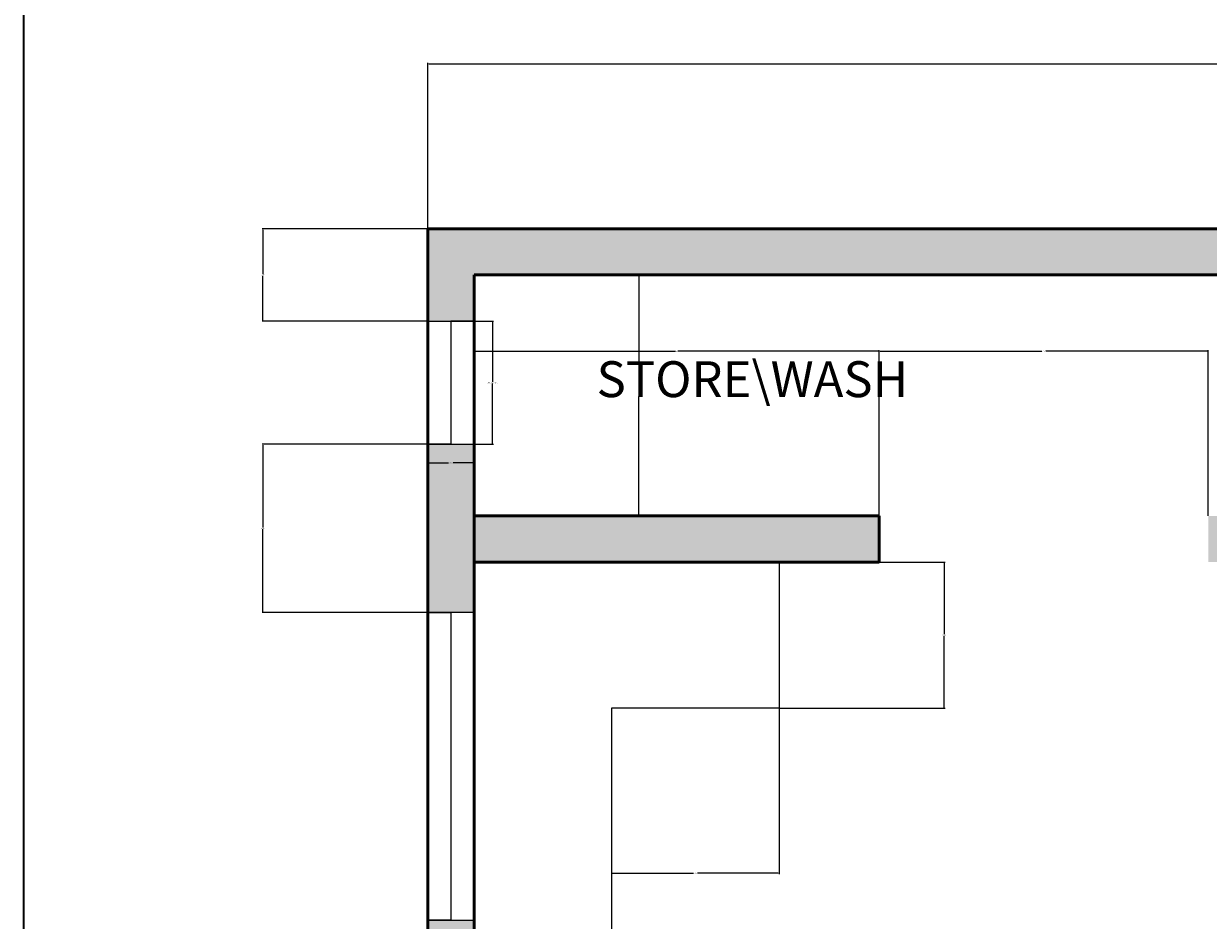
# Model space of a CAD drawing. Units: inches. Extents: x 1676 to 2199, y 1657 to 2783.
# Tile 6 of 10: x 1676 to 1907, y 2206 to 2381. Entities that reach past the tile are written whole.
import ezdxf

# ---------------------------------------------------------------- set-up
doc = ezdxf.new("R2010")
doc.units = ezdxf.units.IN
for name, color, linetype, lineweight in [('A-ANNO-DIMS', 2, 'Continuous', 18), ('A-ANNO-TTLB', 7, 'Continuous', 35), ('A-AREA-IDEN', 7, 'Continuous', 18), ('A-FLOR-CASE', 7, 'Continuous', 25), ('A-GLAZ', 4, 'Continuous', 18), ('A-WALL', 7, 'Continuous', 50)]:
    doc.layers.add(name, color=color, linetype=linetype, lineweight=lineweight)
doc.layers.add('A-WALL-PATT', color=251, linetype='Continuous', lineweight=13, true_color=0x636466)
doc.styles.get("Standard").update_dxf_attribs({"font": 'arial.ttf'})
doc.dimstyles.get("Standard").update_dxf_attribs({"dimtxt": 0.18, "dimasz": 0.18, "dimexe": 0.18, "dimexo": 0.0625, "dimgap": 0.09, "dimtad": 0, "dimtih": 1, "dimtoh": 1, "dimdec": 4, "dimzin": 0, "dimdsep": 46, "dimtxsty": 'Standard', "dimcen": 0.09, "dimadec": 0, "dimazin": 0, "dimtfac": 1, "dimtdec": 4, "dimtofl": 0, "dimtmove": 0, "dimatfit": 3, "dimfxl": 1, "dimtolj": 1, "dimtzin": 0, "dimarcsym": 0})

# ---------------------------------------------------------------- blocks, each defined once
blk = doc.blocks.new('WIN-24')
for p, q in [((0, 0), (9, 0)), ((9, 0), (4.5, 0)), ((4.5, 0), (4.5, -24)), ((4.5, -24), (0, -24)), ((0, -24), (9, -24))]:
    blk.add_line(p, q)
blk = doc.blocks.new('*D9')
at = {"layer": 'A-ANNO-DIMS', "color": 0, "lineweight": -2, "transparency": 16777216}
for p, q in [((1764.14, 2323.07), (1767.85, 2323.07)), ((1767.67, 2322.89), (1767.67, 2311.26)), ((1767.67, 2299.25), (1767.67, 2310.89)), ((1764.14, 2299.07), (1767.85, 2299.07))]:
    blk.add_line(p, q, dxfattribs=at)
at = {"layer": 'A-ANNO-DIMS', "color": 0, "transparency": 16777216}
for points in [[(1767.64, 2322.89), (1767.7, 2322.89), (1767.67, 2323.07)], [(1767.64, 2299.25), (1767.7, 2299.25), (1767.67, 2299.07)]]:
    blk.add_solid(points, dxfattribs=at)
at = {"layer": 'Defpoints', "color": 0, "transparency": 16777216}
for p in [(1764.07, 2323.07), (1767.67, 2323.07), (1764.07, 2299.07)]:
    blk.add_point(p, dxfattribs=at)
at = {"layer": 'A-ANNO-DIMS', "color": 0, "transparency": 16777216, "insert": (1767.67, 2311.07), "char_height": 0.18, "attachment_point": 5}
blk.add_mtext('\\A1;WINDOW 24 TYP.', dxfattribs=at)
blk = doc.blocks.new('*D10')
at = {"layer": 'A-ANNO-DIMS', "color": 0, "lineweight": -2, "transparency": 16777216}
for p, q in [((1755.07, 2299.01), (1755.07, 2295.29)), ((1764.07, 2299.01), (1764.07, 2295.29)), ((1755.25, 2295.47), (1759.12, 2295.47)), ((1763.89, 2295.47), (1760.03, 2295.47))]:
    blk.add_line(p, q, dxfattribs=at)
at = {"layer": 'A-ANNO-DIMS', "color": 0, "transparency": 16777216}
for points in [[(1755.25, 2295.5), (1755.25, 2295.44), (1755.07, 2295.47)], [(1763.89, 2295.5), (1763.89, 2295.44), (1764.07, 2295.47)]]:
    blk.add_solid(points, dxfattribs=at)
at = {"layer": 'Defpoints', "color": 0, "transparency": 16777216}
for p in [(1755.07, 2299.07), (1764.07, 2299.07), (1764.07, 2295.47)]:
    blk.add_point(p, dxfattribs=at)
at = {"layer": 'A-ANNO-DIMS', "color": 0, "transparency": 16777216, "insert": (1759.57, 2295.47), "char_height": 0.18, "attachment_point": 5}
blk.add_mtext('\\A1;9 TYP.', dxfattribs=at)
blk = doc.blocks.new('*D19')
at = {"layer": 'A-ANNO-DIMS', "color": 0, "lineweight": -2, "transparency": 16777216}
for p, q in [((1755.07, 2341.15), (1755.07, 2373.42)), ((1755.25, 2373.24), (1948.29, 2373.24)), ((2141.89, 2373.24), (1948.86, 2373.24)), ((2142.07, 2341.15), (2142.07, 2373.42))]:
    blk.add_line(p, q, dxfattribs=at)
at = {"layer": 'A-ANNO-DIMS', "color": 0, "transparency": 16777216}
for points in [[(1755.25, 2373.27), (1755.25, 2373.21), (1755.07, 2373.24)], [(2141.89, 2373.27), (2141.89, 2373.21), (2142.07, 2373.24)]]:
    blk.add_solid(points, dxfattribs=at)
at = {"layer": 'Defpoints', "color": 0, "transparency": 16777216}
for p in [(2142.07, 2373.24), (1755.07, 2341.09), (2142.07, 2341.09)]:
    blk.add_point(p, dxfattribs=at)
at = {"layer": 'A-ANNO-DIMS', "color": 0, "transparency": 16777216, "insert": (1948.57, 2373.24), "char_height": 0.18, "attachment_point": 5}
blk.add_mtext('\\A1;387', dxfattribs=at)
blk = doc.blocks.new('*D28')
at = {"layer": 'A-ANNO-DIMS', "color": 0, "lineweight": -2, "transparency": 16777216}
for p, q in [((1755.01, 2299.07), (1722.74, 2299.07)), ((1722.92, 2298.89), (1722.92, 2282.85)), ((1722.92, 2266.44), (1722.92, 2282.49)), ((1755.01, 2266.26), (1722.74, 2266.26))]:
    blk.add_line(p, q, dxfattribs=at)
at = {"layer": 'A-ANNO-DIMS', "color": 0, "transparency": 16777216}
for points in [[(1722.89, 2298.89), (1722.95, 2298.89), (1722.92, 2299.07)], [(1722.89, 2266.44), (1722.95, 2266.44), (1722.92, 2266.26)]]:
    blk.add_solid(points, dxfattribs=at)
at = {"layer": 'Defpoints', "color": 0, "transparency": 16777216}
for p in [(1722.92, 2299.07), (1755.07, 2299.07), (1755.07, 2266.26)]:
    blk.add_point(p, dxfattribs=at)
at = {"layer": 'A-ANNO-DIMS', "color": 0, "transparency": 16777216, "insert": (1722.92, 2282.67), "char_height": 0.18, "attachment_point": 5}
blk.add_mtext('\\A1;32.814', dxfattribs=at)
blk = doc.blocks.new('*D29')
at = {"layer": 'A-ANNO-DIMS', "color": 0, "lineweight": -2, "transparency": 16777216}
for p, q in [((1755.01, 2341.09), (1722.74, 2341.09)), ((1722.92, 2340.91), (1722.92, 2332.26)), ((1722.92, 2323.25), (1722.92, 2331.9)), ((1755.01, 2323.07), (1722.74, 2323.07))]:
    blk.add_line(p, q, dxfattribs=at)
at = {"layer": 'A-ANNO-DIMS', "color": 0, "transparency": 16777216}
for points in [[(1722.89, 2340.91), (1722.95, 2340.91), (1722.92, 2341.09)], [(1722.89, 2323.25), (1722.95, 2323.25), (1722.92, 2323.07)]]:
    blk.add_solid(points, dxfattribs=at)
at = {"layer": 'Defpoints', "color": 0, "transparency": 16777216}
for p in [(1722.92, 2341.09), (1755.07, 2341.09), (1755.07, 2323.07)]:
    blk.add_point(p, dxfattribs=at)
at = {"layer": 'A-ANNO-DIMS', "color": 0, "transparency": 16777216, "insert": (1722.92, 2332.08), "char_height": 0.18, "attachment_point": 5}
blk.add_mtext('\\A1;18.013', dxfattribs=at)
blk = doc.blocks.new('*D37')
at = {"layer": 'A-ANNO-DIMS', "color": 0, "lineweight": -2, "transparency": 16777216}
for p, q in [((1764.07, 2285.15), (1764.07, 2317.42)), ((1764.25, 2317.24), (1803.36, 2317.24)), ((1842.89, 2317.24), (1803.79, 2317.24)), ((1843.07, 2285.15), (1843.07, 2317.42))]:
    blk.add_line(p, q, dxfattribs=at)
at = {"layer": 'A-ANNO-DIMS', "color": 0, "transparency": 16777216}
for points in [[(1764.25, 2317.27), (1764.25, 2317.21), (1764.07, 2317.24)], [(1842.89, 2317.27), (1842.89, 2317.21), (1843.07, 2317.24)]]:
    blk.add_solid(points, dxfattribs=at)
at = {"layer": 'Defpoints', "color": 0, "transparency": 16777216}
for p in [(1843.07, 2317.24), (1764.07, 2285.09), (1843.07, 2285.09)]:
    blk.add_point(p, dxfattribs=at)
at = {"layer": 'A-ANNO-DIMS', "color": 0, "transparency": 16777216, "insert": (1803.57, 2317.24), "char_height": 0.18, "attachment_point": 5}
blk.add_mtext('\\A1;79', dxfattribs=at)
blk = doc.blocks.new('*D38')
at = {"layer": 'A-ANNO-DIMS', "color": 0, "lineweight": -2, "transparency": 16777216}
for p, q in [((1843.07, 2285.15), (1843.07, 2317.42)), ((1843.25, 2317.24), (1874.77, 2317.24)), ((1907.07, 2317.24), (1875.56, 2317.24)), ((1907.25, 2285.15), (1907.25, 2317.42))]:
    blk.add_line(p, q, dxfattribs=at)
at = {"layer": 'A-ANNO-DIMS', "color": 0, "transparency": 16777216}
for points in [[(1843.25, 2317.27), (1843.25, 2317.21), (1843.07, 2317.24)], [(1907.07, 2317.27), (1907.07, 2317.21), (1907.25, 2317.24)]]:
    blk.add_solid(points, dxfattribs=at)
at = {"layer": 'Defpoints', "color": 0, "transparency": 16777216}
for p in [(1907.25, 2317.24), (1843.07, 2285.09), (1907.25, 2285.09)]:
    blk.add_point(p, dxfattribs=at)
at = {"layer": 'A-ANNO-DIMS', "color": 0, "transparency": 16777216, "insert": (1875.16, 2317.24), "char_height": 0.18, "attachment_point": 5}
blk.add_mtext('\\A1;64.17', dxfattribs=at)
blk = doc.blocks.new('*D39')
at = {"layer": 'A-ANNO-DIMS', "color": 0, "lineweight": -2, "transparency": 16777216}
for p, q in [((1764.13748, 2332.087058), (1796.40498, 2332.087058)), ((1796.22498, 2331.907058), (1796.22498, 2308.767058)), ((1796.22498, 2285.267058), (1796.22498, 2308.407058)), ((1764.13748, 2285.087058), (1796.40498, 2285.087058))]:
    blk.add_line(p, q, dxfattribs=at)
at = {"layer": 'A-ANNO-DIMS', "color": 0, "transparency": 16777216}
for points in [[(1796.19498, 2331.907058), (1796.25498, 2331.907058), (1796.22498, 2332.087058)], [(1796.19498, 2285.267058), (1796.25498, 2285.267058), (1796.22498, 2285.087058)]]:
    blk.add_solid(points, dxfattribs=at)
at = {"layer": 'Defpoints', "color": 0, "transparency": 16777216}
for p in [(1764.07498, 2332.087058), (1764.07498, 2285.087058), (1796.22498, 2285.087058)]:
    blk.add_point(p, dxfattribs=at)
at = {"layer": 'A-ANNO-DIMS', "color": 0, "transparency": 16777216, "insert": (1796.22498, 2308.587058), "char_height": 0.18, "attachment_point": 5}
blk.add_mtext('\\A1;47', dxfattribs=at)
blk = doc.blocks.new('*D52')
at = {"layer": 'A-ANNO-DIMS', "color": 0, "lineweight": -2, "transparency": 16777216}
for p, q in [((1790.9, 2247.53), (1790.9, 2215.27)), ((1823.59, 2247.53), (1823.59, 2215.27)), ((1791.08, 2215.45), (1806.85, 2215.45)), ((1823.41, 2215.45), (1807.64, 2215.45))]:
    blk.add_line(p, q, dxfattribs=at)
at = {"layer": 'A-ANNO-DIMS', "color": 0, "transparency": 16777216}
for points in [[(1791.08, 2215.48), (1791.08, 2215.42), (1790.9, 2215.45)], [(1823.41, 2215.48), (1823.41, 2215.42), (1823.59, 2215.45)]]:
    blk.add_solid(points, dxfattribs=at)
at = {"layer": 'Defpoints', "color": 0, "transparency": 16777216}
for p in [(1790.9, 2247.6), (1823.59, 2247.6), (1790.9, 2215.45)]:
    blk.add_point(p, dxfattribs=at)
at = {"layer": 'A-ANNO-DIMS', "color": 0, "transparency": 16777216, "insert": (1807.24, 2215.45), "char_height": 0.18, "attachment_point": 5}
blk.add_mtext('\\A1;32.69', dxfattribs=at)
blk = doc.blocks.new('*D53')
at = {"layer": 'A-ANNO-DIMS', "color": 0, "lineweight": -2, "transparency": 16777216}
for p, q in [((1823.65, 2276.09), (1855.92, 2276.09)), ((1855.74, 2275.91), (1855.74, 2262.02)), ((1855.74, 2247.78), (1855.74, 2261.66)), ((1823.65, 2247.6), (1855.92, 2247.6))]:
    blk.add_line(p, q, dxfattribs=at)
at = {"layer": 'A-ANNO-DIMS', "color": 0, "transparency": 16777216}
for points in [[(1855.71, 2275.91), (1855.77, 2275.91), (1855.74, 2276.09)], [(1855.71, 2247.78), (1855.77, 2247.78), (1855.74, 2247.6)]]:
    blk.add_solid(points, dxfattribs=at)
at = {"layer": 'Defpoints', "color": 0, "transparency": 16777216}
for p in [(1823.59, 2276.09), (1823.59, 2247.6), (1855.74, 2247.6)]:
    blk.add_point(p, dxfattribs=at)
at = {"layer": 'A-ANNO-DIMS', "color": 0, "transparency": 16777216, "insert": (1855.74, 2261.84), "char_height": 0.18, "attachment_point": 5}
blk.add_mtext('\\A1;28.49', dxfattribs=at)

msp = doc.modelspace()

# ---------------------------------------------------------------- hatches: boundary and pattern name
at = {"layer": 'A-WALL-PATT'}
h = msp.add_hatch(color=256, dxfattribs=at)
h.dxf.hatch_style = 1
h.paths.add_polyline_path([(1945.4216, 2336.5871), (1945.4216, 2341.0871), (1755.075, 2341.0871), (1755.075, 2323.0739), (1764.075, 2323.0739), (1764.075, 2332.0871), (1945.4216, 2332.0871)])
h.paths.add_polyline_path([(1764.075, 2299.0739), (1755.075, 2299.0739), (1755.075, 2266.2601), (1759.575, 2266.2601), (1764.075, 2266.2601)])
h.paths.add_polyline_path([(1843.075, 2285.0871), (1764.075, 2285.0871), (1764.075, 2276.0871), (1843.075, 2276.0871)])
h.paths.add_polyline_path([(1931.075, 2332.0871), (1922.075, 2332.0871), (1922.075, 2285.0871), (1907.247, 2285.0871), (1907.247, 2276.0871), (1922.075, 2276.0871), (1922.075, 2263.0871), (1922.075, 2214.434), (1922.075, 2183.2198), (1931.075, 2183.2198), (1931.075, 2214.434), (1931.075, 2227.0871), (1991.075, 2227.0871), (1991.075, 2176.0871), (1991.075, 2167.0871), (2000.075, 2167.0871), (2133.075, 2167.0871), (2133.075, 2176.0871), (2000.075, 2176.0871), (2000.075, 2245.3418), (1995.575, 2245.3418), (1991.075, 2245.3418), (1991.075, 2236.0871), (1931.075, 2236.0871)])
h.paths.add_polyline_path([(2000.075, 2332.0871), (1991.075, 2332.0871), (1991.075, 2285.0871), (1991.075, 2274.6339), (2000.075, 2274.6339), (2000.075, 2285.0871)], flags=17)
h.paths.add_polyline_path([(2142.075, 2341.0871), (1969.4216, 2341.0871), (1969.4216, 2332.0871), (2133.075, 2332.0871), (2133.075, 2298.2101), (2142.075, 2298.2101)])
h.paths.add_polyline_path([(2142.075, 1844.9908), (2133.075, 1844.9908), (2133.075, 1790.0871), (2061.2106, 1790.0871), (2061.2106, 1781.0871), (2142.075, 1781.0871)])
h.paths.add_polyline_path([(2001.2106, 1790.0871), (1966.075, 1790.0871), (1966.075, 1957.0871), (1973.4183, 1957.0871), (1973.4183, 1966.0871), (1966.075, 1966.0871), (1966.075, 1983.1515), (1957.075, 1983.1515), (1957.075, 1899.0871), (1946.8789, 1899.0871), (1946.8789, 1890.0871), (1957.075, 1890.0871), (1957.075, 1781.0871), (2001.2106, 1781.0871), (2001.2106, 1785.5871)])
h.paths.add_polyline_path([(1876.3163, 1894.5871), (1876.3163, 1899.0871), (1820.9237, 1899.0871), (1820.9237, 1890.0871), (1876.3163, 1890.0871)])
h.paths.add_polyline_path([(1764.075, 2093.9207), (1759.575, 2093.9207), (1755.075, 2093.9207), (1755.075, 2019.5723), (1764.075, 2019.5723)])
h.paths.add_polyline_path([(1878.3926, 2083.0871), (1764.075, 2083.0871), (1764.075, 2074.0871), (1878.3926, 2074.0871)])
h.paths.add_polyline_path([(1764.075, 1959.5723), (1755.075, 1959.5723), (1755.075, 1890.0871), (1784.9237, 1890.0871), (1784.9237, 1894.5871), (1784.9237, 1899.0871), (1764.075, 1899.0871)])
h.paths.add_polyline_path([(2133.075, 2047.0871), (2000.075, 2047.0871), (1966.075, 2047.0871), (1957.075, 2047.0871), (1938.4046, 2047.0871), (1938.4046, 2038.0871), (1957.075, 2038.0871), (1957.075, 2026.1604), (1966.075, 2026.1604), (1966.075, 2038.0871), (2039.075, 2038.0871), (2039.075, 2011.4216), (2048.075, 2011.4216), (2048.075, 2038.0871), (2133.075, 2038.0871)])
h.paths.add_polyline_path([(2133.075, 1966.0871), (2048.075, 1966.0871), (2048.075, 1972.5045), (2039.075, 1972.5045), (2039.075, 1966.0871), (2025.1075, 1966.0871), (2025.1075, 1957.0871), (2133.075, 1957.0871)])
h.paths.add_polyline_path([(1764.075, 2206.2601), (1755.075, 2206.2601), (1755.075, 2153.9207), (1764.075, 2153.9207)])

# ---------------------------------------------------------------- linework, layer by layer
at = {"layer": 'A-ANNO-TTLB'}
msp.add_lwpolyline([(1676.2722, 2782.5054), (2199.4461, 2782.5054), (2199.4461, 1657.2705), (1676.2722, 1657.2705)], close=True, dxfattribs=at)
at = {"layer": 'A-FLOR-CASE'}
for p, q in [((1823.5884, 2276.0871), (1823.5884, 2247.5974)), ((1823.5884, 2247.5974), (1790.8966, 2247.5974)), ((1790.8966, 2247.5974), (1790.8966, 2083.0871))]:
    msp.add_line(p, q, dxfattribs=at)
at = {"layer": 'A-GLAZ'}
for p, q in [((1764.075, 2266.2601), (1755.075, 2266.2601)), ((1755.075, 2266.2601), (1759.575, 2266.2601)), ((1759.575, 2266.2601), (1759.575, 2206.2601)), ((1759.575, 2206.2601), (1755.075, 2206.2601)), ((1755.075, 2206.2601), (1764.075, 2206.2601))]:
    msp.add_line(p, q, dxfattribs=at)
at = {"layer": 'A-WALL'}
for p, q in [((1755.075, 2341.0871), (2142.075, 2341.0871)), ((1755.075, 2341.0871), (1755.075, 1890.0871)), ((1764.075, 2332.0871), (2133.075, 2332.0871)), ((1764.075, 2332.0871), (1764.075, 1899.0871)), ((1764.075, 2285.0871), (1843.075, 2285.0871)), ((1843.075, 2285.0871), (1843.075, 2276.0871)), ((1764.075, 2276.0871), (1843.075, 2276.0871))]:
    msp.add_line(p, q, dxfattribs=at)

# ---------------------------------------------------------------- block references
at = {"layer": 'A-GLAZ'}
msp.add_blockref('WIN-24', (1755.075, 2323.0739), dxfattribs=at)

# ---------------------------------------------------------------- texts
at = {"layer": 'A-AREA-IDEN', "insert": (1787.9804, 2315.2599), "char_height": 7, "attachment_point": 1}
msp.add_mtext_dynamic_manual_height_columns('STORE\\\\WASH', width=162.291606, gutter_width=12.5, heights=[0], dxfattribs=at)

# ---------------------------------------------------------------- dimensions: what is measured, and where the dimension line sits
at = {"layer": 'A-ANNO-DIMS'}
for base, p1, p2, override, picture, middle in [((2142.075, 2373.2371), (1755.075, 2341.0871), (2142.075, 2341.0871), {"dimdec": 0, "dimlfac": 1, "dimrnd": 0, "dimzin": 0, "dimdsep": 46, "dimlunit": 2}, '*D19', (1948.575, 2373.2371)), ((1843.075, 2317.2371), (1764.075, 2285.0871), (1843.075, 2285.0871), {"dimdec": 0, "dimlfac": 1, "dimrnd": 0, "dimzin": 0, "dimdsep": 46, "dimlunit": 2}, '*D37', (1803.575, 2317.2371)), ((1907.247, 2317.2371), (1843.075, 2285.0871), (1907.247, 2285.0871), {"dimdec": 2, "dimlfac": 1, "dimrnd": 0, "dimzin": 0, "dimdsep": 46, "dimlunit": 2}, '*D38', (1875.161, 2317.2371))]:
    dim = msp.add_linear_dim(base=base, p1=p1, p2=p2, dimstyle='Standard', override=override, dxfattribs=at)
    dim.commit()
    dim.dimension.update_dxf_attribs({"geometry": picture, "text_midpoint": middle})
for base, p1, p2, angle, override, picture, middle in [((1722.925, 2341.0871), (1755.075, 2323.0739), (1755.075, 2341.0871), 90, {"dimdec": 3, "dimlfac": 1, "dimrnd": 0, "dimzin": 0, "dimdsep": 46, "dimlunit": 2}, '*D29', (1722.925, 2332.0805)), ((1796.225, 2285.0871), (1764.075, 2332.0871), (1764.075, 2285.0871), 270, {"dimdec": 0, "dimlfac": 1, "dimrnd": 0, "dimzin": 0, "dimdsep": 46, "dimlunit": 2}, '*D39', (1796.225, 2308.5871)), ((1722.925, 2299.0739), (1755.075, 2266.2601), (1755.075, 2299.0739), 90, {"dimdec": 3, "dimlfac": 1, "dimrnd": 0, "dimzin": 0, "dimdsep": 46, "dimlunit": 2}, '*D28', (1722.925, 2282.667)), ((1855.7384, 2247.5974), (1823.5884, 2276.0871), (1823.5884, 2247.5974), 270, {"dimdec": 2, "dimlfac": 1, "dimrnd": 0, "dimzin": 0, "dimdsep": 46, "dimlunit": 2}, '*D53', (1855.7384, 2261.8422)), ((1790.8966, 2215.4474), (1823.5884, 2247.5974), (1790.8966, 2247.5974), 180, {"dimdec": 2, "dimlfac": 1, "dimrnd": 0, "dimzin": 0, "dimdsep": 46, "dimlunit": 2}, '*D52', (1807.2425, 2215.4474))]:
    dim = msp.add_linear_dim(base=base, p1=p1, p2=p2, angle=angle, dimstyle='Standard', override=override, dxfattribs=at)
    dim.commit()
    dim.dimension.update_dxf_attribs({"geometry": picture, "text_midpoint": middle})
dim = msp.add_linear_dim(base=(1767.675, 2323.0739), p1=(1764.075, 2299.0739), p2=(1764.075, 2323.0739), angle=90, text='WINDOW <> TYP.', dimstyle='Standard', override={"dimdec": 0, "dimlfac": 1, "dimrnd": 0, "dimzin": 0, "dimdsep": 46, "dimlunit": 2}, dxfattribs=at)
dim.commit()
dim.dimension.update_dxf_attribs({"geometry": '*D9', "text_midpoint": (1767.675, 2311.0739)})
dim = msp.add_linear_dim(base=(1764.075, 2295.4739), p1=(1755.075, 2299.0739), p2=(1764.075, 2299.0739), text='<> TYP.', dimstyle='Standard', override={"dimdec": 0, "dimlfac": 1, "dimrnd": 0, "dimzin": 0, "dimdsep": 46, "dimlunit": 2}, dxfattribs=at)
dim.commit()
dim.dimension.update_dxf_attribs({"geometry": '*D10', "text_midpoint": (1759.575, 2295.4739)})

doc.saveas('drawing.dxf')
